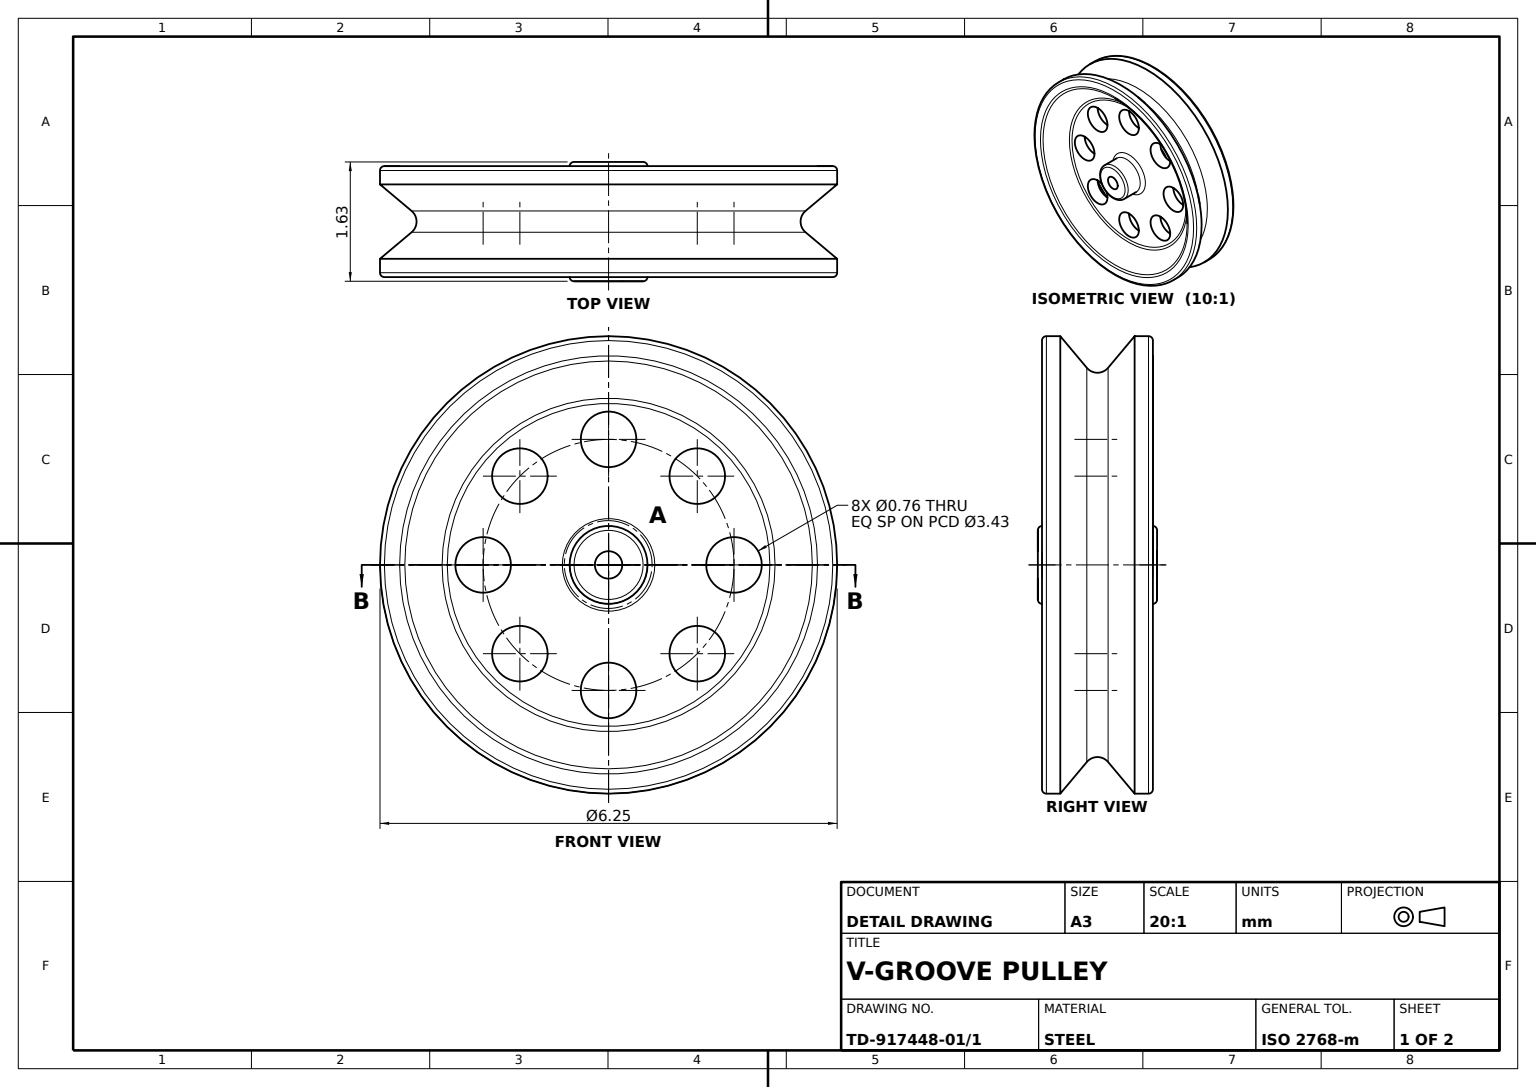
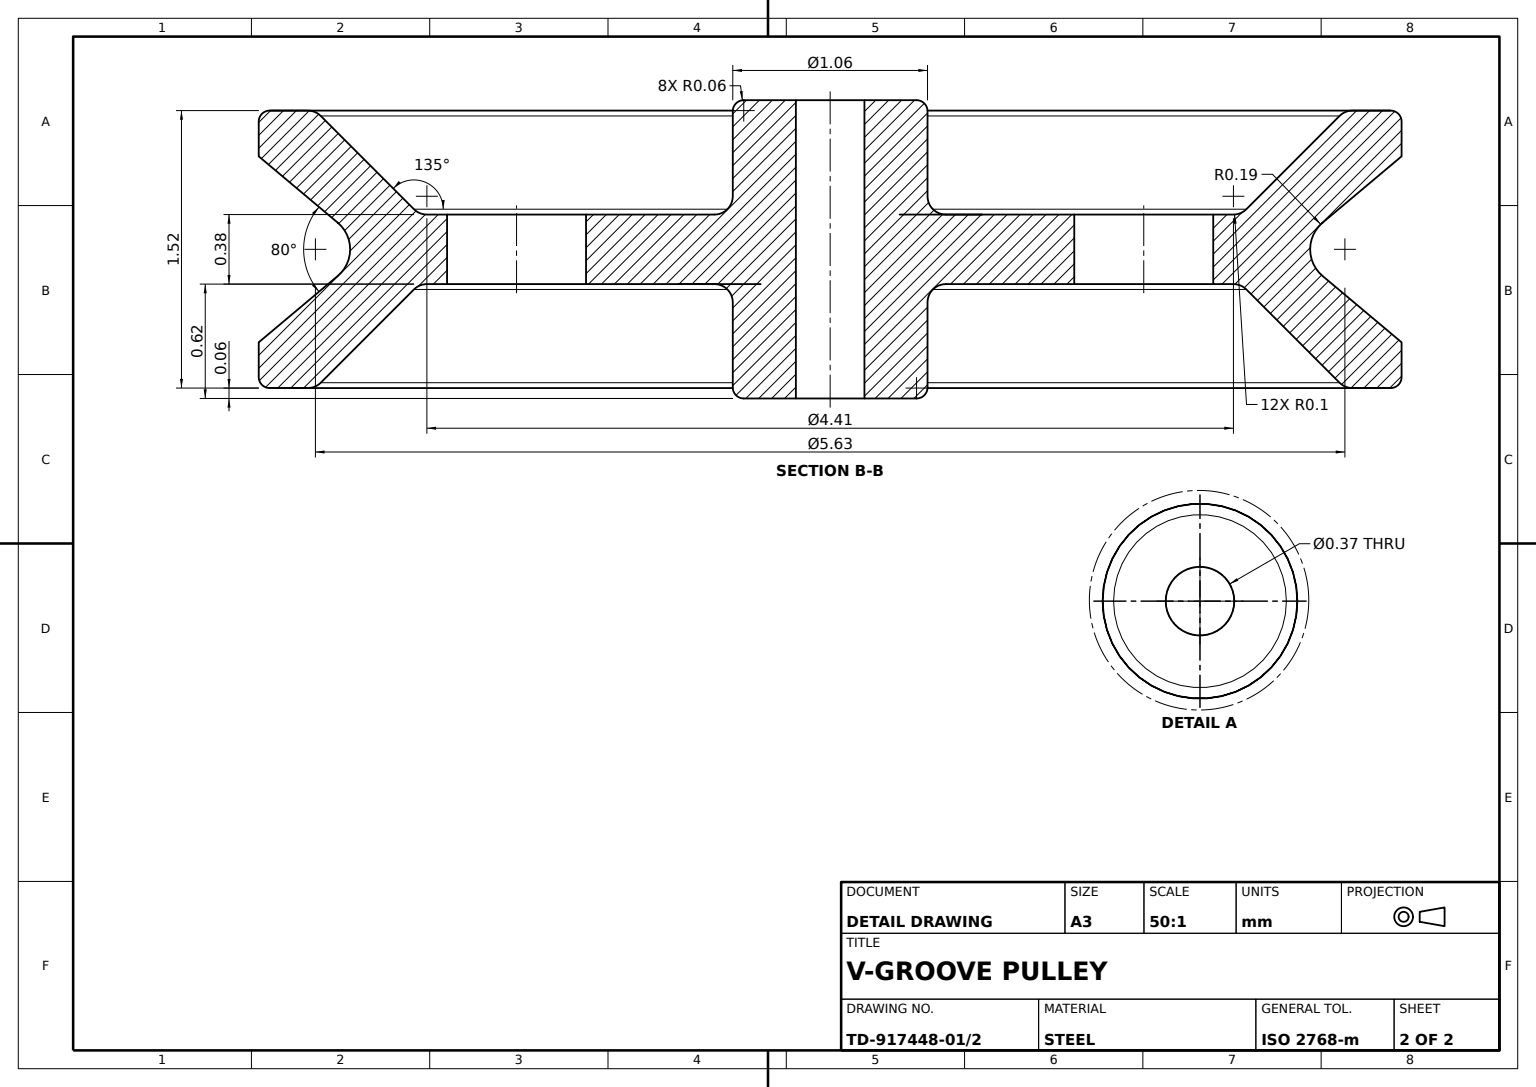
from build123d import *

# Parameters (mm, degrees)
EDGE_FILLETS_R0_06_SET_1_R      = 0.06
WEB_FILLET_R0_1_R               = 0.1
EDGE_FILLETS_R0_06_SET_2_R      = 0.06
BOLT_HOLE_SKETCH_R              = 0.38
BOLT_HOLE_0_76_DEPTH            = 5.532248476
BOLT_CIRCLE_HOLES_8X_0_76_COUNT = 8


with BuildPart() as part:
    # Pulley Profile Sketch → Pulley Body Revolve (revolve)
    with BuildSketch(Plane.XY, mode=Mode.PRIVATE) as pulley_body_revolve_sk:
        with BuildLine():
            Line((-0.815, 0.1875), (0.815, 0.1875))
            Line((0.815, 0.1875), (0.815, 0.5325))
            Line((0.815, 0.5325), (0.19, 0.5325))
            Line((0.19, 0.5325), (0.19, 2.246851729))
            Line((0.19, 2.246851729), (0.758148271, 2.815))
            Line((0.758148271, 2.815), (0.758148271, 3.125))
            Line((0.758148271, 3.125), (0.508148271, 3.125))
            Line((0.508148271, 3.125), (0.145548444, 2.692870354))
            ThreePointArc((0.145548444, 2.692870354), (0, 2.625), (-0.145548444, 2.692870354))
            Line((-0.145548444, 2.692870354), (-0.508148271, 3.125))
            Line((-0.508148271, 3.125), (-0.758148271, 3.125))
            Line((-0.758148271, 3.125), (-0.758148271, 2.815))
            Line((-0.758148271, 2.815), (-0.19, 2.246851729))
            Line((-0.19, 2.246851729), (-0.19, 0.5325))
            Line((-0.19, 0.5325), (-0.815, 0.5325))
            Line((-0.815, 0.5325), (-0.815, 0.1875))
        make_face()
    revolve(pulley_body_revolve_sk.sketch.rotate(Axis((0, 0, 0), (1, 0, 0)), 90), axis=Axis((0, 0, 0), (1, 0, 0)))

    # Edge Fillets R0.06 Set 1
    edge_fillets_r0_06_set_1_edges = [part.edges().sort_by_distance(p)[0] for p in [
        (-0.758148271, 0, -3.125),
        (0.758148271, 0, -3.125),
    ]]
    fillet(edge_fillets_r0_06_set_1_edges, radius=EDGE_FILLETS_R0_06_SET_1_R)

    # Web Fillet R0.1
    web_fillet_r0_1_edges = [part.edges().sort_by_distance(p)[0] for p in [
        (-0.19, 0, -0.5325),
        (-0.19, 0, -2.246851729),
        (-0.758148271, 0, -2.815),
        (0.758148271, 0, -2.815),
        (0.19, 0, -2.246851729),
        (0.19, 0, -0.5325),
    ]]
    fillet(web_fillet_r0_1_edges, radius=WEB_FILLET_R0_1_R)

    # Edge Fillets R0.06 Set 2
    edge_fillets_r0_06_set_2_edges = [part.edges().sort_by_distance(p)[0] for p in [
        (0.815, 0, -0.5325),
        (-0.815, 0, -0.5325),
    ]]
    fillet(edge_fillets_r0_06_set_2_edges, radius=EDGE_FILLETS_R0_06_SET_2_R)

    # Bolt Hole Sketch → Bolt Hole Ø0.76 (cut, through all)
    with BuildSketch(Plane.ZY.offset(0.19)):
        with Locations((0, 1.715)):
            Circle(BOLT_HOLE_SKETCH_R)
    bolt_hole_0_76 = extrude(amount=-BOLT_HOLE_0_76_DEPTH, mode=Mode.SUBTRACT)

    # Bolt Circle Holes 8xØ0.76: Bolt Hole Ø0.76 ×8 about axis
    bolt_circle_holes_8x_0_76_axis = Axis((0, 0, 0), (1, 0, 0))
    for i in range(1, BOLT_CIRCLE_HOLES_8X_0_76_COUNT):
        add(bolt_hole_0_76.rotate(bolt_circle_holes_8x_0_76_axis, i * 360 / BOLT_CIRCLE_HOLES_8X_0_76_COUNT), mode=Mode.SUBTRACT)


solid = part.part
